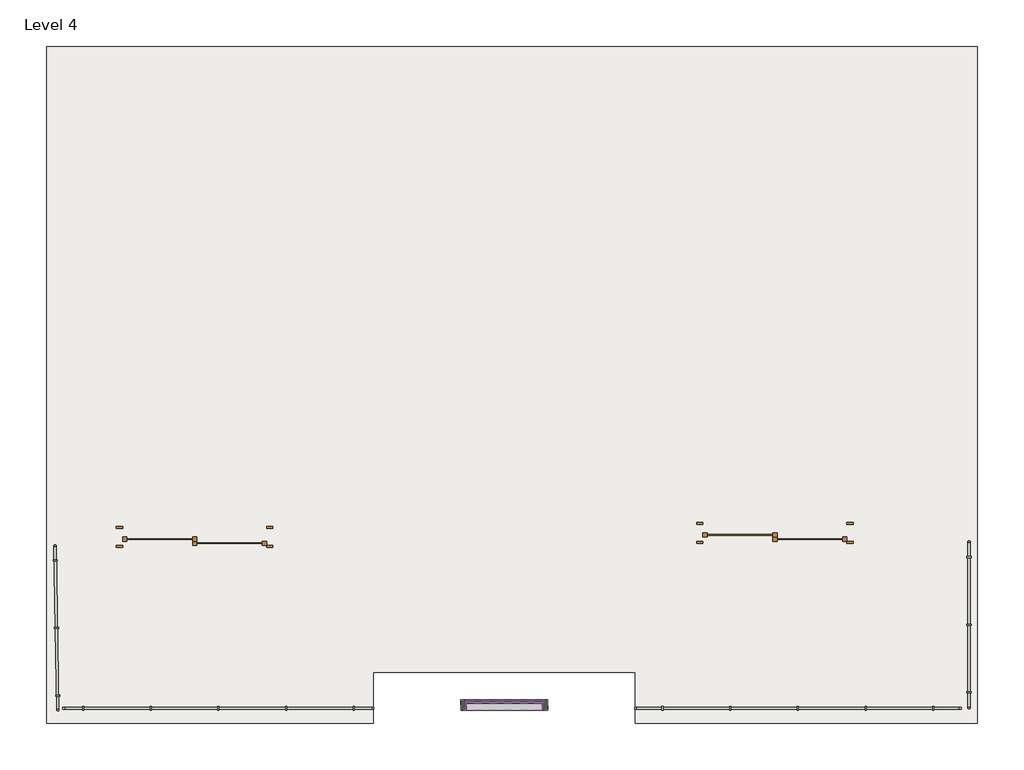
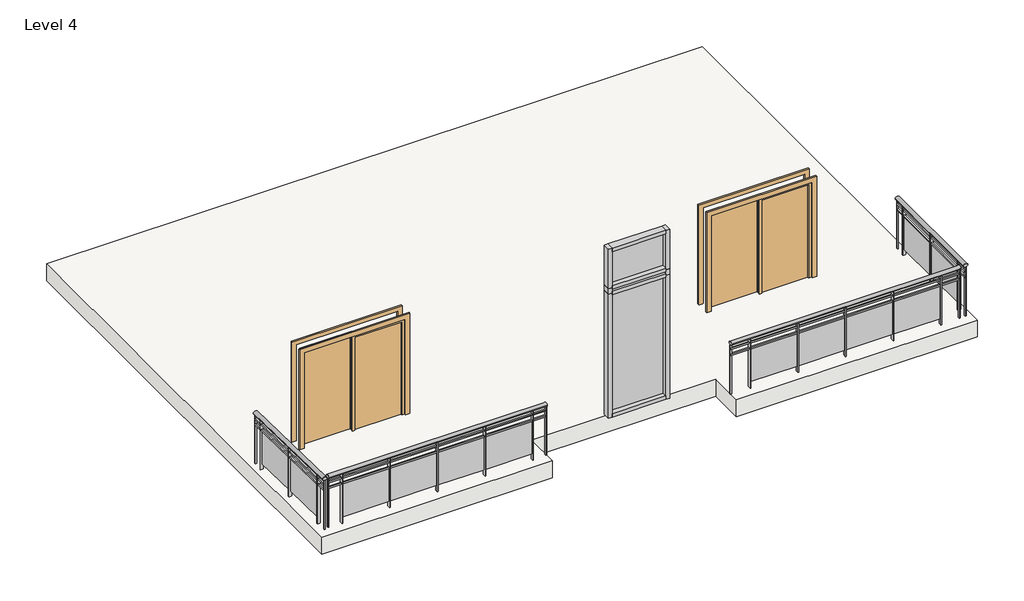
# One storey: 10 members, 4 railings, 3 plates, 2 doors, 1 roof.
"""IFC4 building model written with IfcOpenShell, lengths in millimetres."""

from ifc_helpers import new_model, si_unit, point, frame, origin, place, context, project, spatial, polyline, ellipse_curve, trimmed, outline, extrude, transform, mapped, element, save
from ifc_brep_helpers import plane_surface, extruded_surface, advanced_brep
from components import door_076b30e0, member_d1708325, member_fb13da3b, member_73c23c35, member_410c6227, member_ae70dd35, system_panel_glazed_14bb7e7b, system_panel_glazed_8073c085, system_panel_glazed_7d1a27c5

model = new_model("IFC4")

# Units and contexts
model_context = context("Model", 3, world=origin())
ifc_project = project(units=[si_unit("LENGTHUNIT", "METRE", prefix="MILLI")], contexts=[model_context])

# Site, building, storey
site = spatial("IfcSite", under=ifc_project)
building = spatial("IfcBuilding", under=site)
storey = spatial("IfcBuildingStorey", under=building, Name="Level 4", Elevation=10972.8)

# Doors
placement = place(None, origin())
door_shape = door_076b30e0(model_context)
element("IfcDoor", 1, ObjectType="Door-Double-Sliding : 68\" x 80\"", at=placement, inside=storey, context=model_context, shape_type="MappedRepresentation", body=[
    mapped(door_shape, transform((-2271.8087885, 3717.6236997, 10972.8), x_axis=(-1.0, 0.0, 0.0), y_axis=(0.0, -1.0, 0.0), z_axis=(0.0, 0.0, 1.0))),
])
element("IfcDoor", 2, ObjectType="Door-Double-Sliding : 68\" x 80\"", at=placement, inside=storey, context=model_context, shape_type="MappedRepresentation", body=[
    mapped(door_shape, transform((-9238.1183714, 3666.8236997, 10972.8), x_axis=(-1.0, 0.0, 0.0), y_axis=(0.0, -1.0, 0.0), z_axis=(0.0, 0.0, 1.0))),
])

# Members
member_shape = member_d1708325(model_context)
element("IfcMember", 3, ObjectType="Rectangular Mullion : 2.5\" x 5\" rectangular", at=placement, inside=storey, context=model_context, shape_type="MappedRepresentation", body=[
    mapped(member_shape, transform((-6041.6537147, 1520.5236997, 13817.6), x_axis=(-1.0, 0.0, 0.0), y_axis=(0.0, -1.0, 0.0), z_axis=(0.0, 0.0, 1.0))),
])
member_2_shape = member_fb13da3b(model_context)
element("IfcMember", 4, ObjectType="Rectangular Mullion : 2.5\" x 5\" rectangular", at=placement, inside=storey, context=model_context, shape_type="MappedRepresentation", body=[
    mapped(member_2_shape, transform((-6041.6537147, 1520.5236997, 13919.2), x_axis=(-1.0, 0.0, 0.0), y_axis=(0.0, -1.0, 0.0), z_axis=(0.0, 0.0, 1.0))),
])
member_3_shape = member_73c23c35(model_context)
element("IfcMember", 5, ObjectType="Rectangular Mullion : 2.5\" x 5\" rectangular", at=placement, inside=storey, context=model_context, shape_type="MappedRepresentation", body=[
    mapped(member_3_shape, transform((-5978.1537147, 1520.5236997, 11582.4), x_axis=(0.0, 0.0, -1.0), y_axis=(0.0, -1.0, 0.0), z_axis=(-1.0, 0.0, 0.0))),
])
member_4_shape = member_410c6227(model_context)
element("IfcMember", 6, ObjectType="Rectangular Mullion : 2.5\" x 5\" rectangular", at=placement, inside=storey, context=model_context, shape_type="MappedRepresentation", body=[
    mapped(member_4_shape, transform((-5063.7537147, 1520.5236997, 13817.6), x_axis=(0.0, 0.0, 1.0), y_axis=(0.0, -1.0, 0.0), z_axis=(1.0, 0.0, 0.0))),
])
element("IfcMember", 7, ObjectType="Rectangular Mullion : 2.5\" x 5\" rectangular", at=placement, inside=storey, context=model_context, shape_type="MappedRepresentation", body=[
    mapped(member_4_shape, transform((-5063.7537147, 1520.5236997, 13919.2), x_axis=(0.0, 0.0, 1.0), y_axis=(0.0, -1.0, 0.0), z_axis=(1.0, 0.0, 0.0))),
])
element("IfcMember", 8, ObjectType="Rectangular Mullion : 2.5\" x 5\" rectangular", at=placement, inside=storey, context=model_context, shape_type="MappedRepresentation", body=[
    mapped(member_3_shape, transform((-5063.7537147, 1520.5236997, 14630.4), x_axis=(0.0, 0.0, 1.0), y_axis=(0.0, -1.0, 0.0), z_axis=(1.0, 0.0, 0.0))),
])
element("IfcMember", 9, ObjectType="Rectangular Mullion : 2.5\" x 5\" rectangular", at=placement, inside=storey, context=model_context, shape_type="MappedRepresentation", body=[
    mapped(member_2_shape, transform((-5000.2537147, 1520.5236997, 13817.6), x_axis=(1.0, 0.0, 0.0), y_axis=(0.0, -1.0, 0.0), z_axis=(0.0, 0.0, -1.0))),
])
element("IfcMember", 10, ObjectType="Rectangular Mullion : 2.5\" x 5\" rectangular", at=placement, inside=storey, context=model_context, shape_type="MappedRepresentation", body=[
    mapped(member_shape, transform((-5000.2537147, 1520.5236997, 11582.4), x_axis=(1.0, 0.0, 0.0), y_axis=(0.0, -1.0, 0.0), z_axis=(0.0, 0.0, -1.0))),
])
member_5_shape = member_ae70dd35(model_context)
element("IfcMember", 11, ObjectType="Rectangular Mullion : 2.5\" x 5\" rectangular", at=placement, inside=storey, context=model_context, shape_type="MappedRepresentation", body=[
    mapped(member_5_shape, transform((-6041.6537147, 1520.5236997, 14630.4), x_axis=(-1.0, 0.0, 0.0), y_axis=(0.0, -1.0, 0.0), z_axis=(0.0, 0.0, 1.0))),
])
element("IfcMember", 12, ObjectType="Rectangular Mullion : 2.5\" x 5\" rectangular", at=placement, inside=storey, context=model_context, shape_type="MappedRepresentation", body=[
    mapped(member_5_shape, transform((-5000.2537147, 1520.5236997, 13919.2), x_axis=(1.0, 0.0, 0.0), y_axis=(0.0, -1.0, 0.0), z_axis=(0.0, 0.0, -1.0))),
])

# Plates
system_panel_glazed_shape = system_panel_glazed_14bb7e7b(model_context)
element("IfcPlate", 13, ObjectType="System Panel : Glazed", at=placement, inside=storey, context=model_context, shape_type="MappedRepresentation", body=[
    mapped(system_panel_glazed_shape, transform((-5520.9537147, 1520.5236997, 11645.9), x_axis=(1.0, 0.0, 0.0), y_axis=(0.0, 1.0, 0.0), z_axis=(0.0, 0.0, 1.0))),
])
system_panel_glazed_2_shape = system_panel_glazed_8073c085(model_context)
element("IfcPlate", 14, ObjectType="System Panel : Glazed", at=placement, inside=storey, context=model_context, shape_type="MappedRepresentation", body=[
    mapped(system_panel_glazed_2_shape, transform((-5520.9537147, 1520.5236997, 13849.35), x_axis=(1.0, 0.0, 0.0), y_axis=(0.0, 1.0, 0.0), z_axis=(0.0, 0.0, 1.0))),
])
system_panel_glazed_3_shape = system_panel_glazed_7d1a27c5(model_context)
element("IfcPlate", 15, ObjectType="System Panel : Glazed", at=placement, inside=storey, context=model_context, shape_type="MappedRepresentation", body=[
    mapped(system_panel_glazed_3_shape, transform((-5520.9537147, 1520.5236997, 13950.95), x_axis=(1.0, 0.0, 0.0), y_axis=(0.0, 1.0, 0.0), z_axis=(0.0, 0.0, 1.0))),
])

# Railings
element("IfcRailing", 16, ObjectType="Glass Panel - Bottom Fill", at=placement, inside=storey, context=model_context, shape_type="SolidModel", body=[
    advanced_brep(
    [(-10812.9183714, 1520.5236997, 12192.0), (-10812.9183714, 1444.3236997, 12192.0), (-7091.896639, 1520.5236997, 12192.0), (-7091.896639, 1444.3236997, 12192.0)],
    [
        (0, 1, ellipse_curve(frame((-10812.9183714, 1482.4236997, 12192.0), z_axis=(-1.0, 0.0, 0.0), x_axis=(0.0, -1.0, 0.0)), 38.1, 28.575)),
        (1, 0, ellipse_curve(frame((-10812.9183714, 1482.4236997, 12192.0), z_axis=(-1.0, 0.0, 0.0), x_axis=(0.0, -1.0, 0.0)), 38.1, 28.575)),
        (2, 3, ellipse_curve(frame((-7091.896639, 1482.4236997, 12192.0), z_axis=(1.0, 0.0, 0.0), x_axis=(0.0, -1.0, 0.0)), 38.1, 28.575)),
        (3, 2, ellipse_curve(frame((-7091.896639, 1482.4236997, 12192.0), z_axis=(1.0, 0.0, 0.0), x_axis=(0.0, -1.0, 0.0)), 38.1, 28.575)),
        (0, 2),
        (3, 1),
    ],
    [
        plane_surface(frame((-10812.9183714, 1482.4236997, 12192.0), z_axis=(-1.0, 0.0, 0.0), x_axis=(0.0, 1.0, 0.0))),
        plane_surface(frame((-7091.896639, 1482.4236997, 12192.0), z_axis=(1.0, 0.0, 0.0), x_axis=(0.0, 1.0, 0.0))),
        extruded_surface(trimmed(ellipse_curve(frame((-7091.896639, 1482.4236997, 12192.0), z_axis=(-1.0, 0.0, 0.0), x_axis=(0.0, -1.0, 0.0)), 38.1, 28.575), [point((-7091.896639, 1520.5236997, 12192.0))], [point((-7091.896639, 1444.3236997, 12192.0))], True, "CARTESIAN"), (-3721.0217323999996, 0.0, 0.0), 3721.0217323999996),
        extruded_surface(trimmed(ellipse_curve(frame((-7091.896639, 1482.4236997, 12192.0), z_axis=(-1.0, 0.0, 0.0), x_axis=(0.0, -1.0, 0.0)), 38.1, 28.575), [point((-7091.896639, 1444.3236997, 12192.0))], [point((-7091.896639, 1520.5236997, 12192.0))], True, "CARTESIAN"), (-3721.0217323999996, 0.0, 0.0), 3721.0217323999996),
    ],
    [
        (0, [[1, 2]]),
        (1, [[3, 4]]),
        (2, [[-1, 5, -4, 6]]),
        (3, [[-2, -6, -3, -5]]),
    ],
),
    extrude(outline(polyline([(-10812.9183714, 1469.7236997), (-10812.9183714, 1495.1236997), (-7091.896639, 1495.1236997), (-7091.896639, 1469.7236997), (-10812.9183714, 1469.7236997)])), frame((0.0, 0.0, 12077.7), z_axis=(0.0, 0.0, 1.0), x_axis=(1.0, 0.0, 0.0)), (0.0, 0.0, 1.0), 25.4),
    extrude(outline(polyline([(-10812.9183714, 1469.7236997), (-10812.9183714, 1495.1236997), (-7091.896639, 1495.1236997), (-7091.896639, 1469.7236997), (-10812.9183714, 1469.7236997)])), frame((0.0, 0.0, 11976.1), z_axis=(0.0, 0.0, 1.0), x_axis=(1.0, 0.0, 0.0)), (0.0, 0.0, 1.0), 25.4),
    extrude(outline(polyline([(-7333.1575052, 1457.0236997), (-7333.1575052, 1507.8236997), (-7320.4575052, 1507.8236997), (-7320.4575052, 1457.0236997), (-7333.1575052, 1457.0236997)])), frame((0.0, 0.0, 11277.6), z_axis=(0.0, 0.0, 1.0), x_axis=(1.0, 0.0, 0.0)), (0.0, 0.0, 1.0), 885.6788223),
    extrude(outline(polyline([(-8139.6075052, 1488.9588567), (-7326.8075052, 1488.9588567), (-7326.8075052, 1482.6088567), (-8139.6075052, 1482.6088567), (-8139.6075052, 1488.9588567)])), frame((0.0, 0.0, 11379.2), z_axis=(0.0, 0.0, 1.0), x_axis=(1.0, 0.0, 0.0)), (0.0, 0.0, 1.0), 596.9),
    extrude(outline(polyline([(-8145.9575052, 1457.0236997), (-8145.9575052, 1507.8236997), (-8133.2575052, 1507.8236997), (-8133.2575052, 1457.0236997), (-8145.9575052, 1457.0236997)])), frame((0.0, 0.0, 11277.6), z_axis=(0.0, 0.0, 1.0), x_axis=(1.0, 0.0, 0.0)), (0.0, 0.0, 1.0), 885.6788223),
    extrude(outline(polyline([(-8952.4075052, 1488.9588567), (-8139.6075052, 1488.9588567), (-8139.6075052, 1482.6088567), (-8952.4075052, 1482.6088567), (-8952.4075052, 1488.9588567)])), frame((0.0, 0.0, 11379.2), z_axis=(0.0, 0.0, 1.0), x_axis=(1.0, 0.0, 0.0)), (0.0, 0.0, 1.0), 596.9),
    extrude(outline(polyline([(-8958.7575052, 1457.0236997), (-8958.7575052, 1507.8236997), (-8946.0575052, 1507.8236997), (-8946.0575052, 1457.0236997), (-8958.7575052, 1457.0236997)])), frame((0.0, 0.0, 11277.6), z_axis=(0.0, 0.0, 1.0), x_axis=(1.0, 0.0, 0.0)), (0.0, 0.0, 1.0), 885.6788223),
    extrude(outline(polyline([(-9765.2075052, 1488.9588567), (-8952.4075052, 1488.9588567), (-8952.4075052, 1482.6088567), (-9765.2075052, 1482.6088567), (-9765.2075052, 1488.9588567)])), frame((0.0, 0.0, 11379.2), z_axis=(0.0, 0.0, 1.0), x_axis=(1.0, 0.0, 0.0)), (0.0, 0.0, 1.0), 596.9),
    extrude(outline(polyline([(-9771.5575052, 1457.0236997), (-9771.5575052, 1507.8236997), (-9758.8575052, 1507.8236997), (-9758.8575052, 1457.0236997), (-9771.5575052, 1457.0236997)])), frame((0.0, 0.0, 11277.6), z_axis=(0.0, 0.0, 1.0), x_axis=(1.0, 0.0, 0.0)), (0.0, 0.0, 1.0), 885.6788223),
    extrude(outline(polyline([(-10578.0075052, 1488.9588567), (-9765.2075052, 1488.9588567), (-9765.2075052, 1482.6088567), (-10578.0075052, 1482.6088567), (-10578.0075052, 1488.9588567)])), frame((0.0, 0.0, 11379.2), z_axis=(0.0, 0.0, 1.0), x_axis=(1.0, 0.0, 0.0)), (0.0, 0.0, 1.0), 596.9),
    extrude(outline(polyline([(-10584.3575052, 1457.0236997), (-10584.3575052, 1507.8236997), (-10571.6575052, 1507.8236997), (-10571.6575052, 1457.0236997), (-10584.3575052, 1457.0236997)])), frame((0.0, 0.0, 11277.6), z_axis=(0.0, 0.0, 1.0), x_axis=(1.0, 0.0, 0.0)), (0.0, 0.0, 1.0), 885.6788223),
    extrude(outline(polyline([(-7104.596639, 1472.8986997), (-7104.596639, 1491.9486997), (-7085.546639, 1491.9486997), (-7085.546639, 1472.8986997), (-7104.596639, 1472.8986997)])), frame((0.0, 0.0, 11277.6), z_axis=(0.0, 0.0, 1.0), x_axis=(1.0, 0.0, 0.0)), (0.0, 0.0, 1.0), 885.6788223),
    extrude(outline(polyline([(-10819.2683714, 1472.8986997), (-10819.2683714, 1491.9486997), (-10800.2183714, 1491.9486997), (-10800.2183714, 1472.8986997), (-10819.2683714, 1472.8986997)])), frame((0.0, 0.0, 11277.6), z_axis=(0.0, 0.0, 1.0), x_axis=(1.0, 0.0, 0.0)), (0.0, 0.0, 1.0), 885.6788223),
])
element("IfcRailing", 17, ObjectType="Glass Panel - Bottom Fill", at=placement, inside=storey, context=model_context, shape_type="SolidModel", body=[
    advanced_brep(
    [(-3948.2087885, 1520.5236997, 12192.0), (-3948.2087885, 1444.3236997, 12192.0), (-43.3183714, 1520.5236997, 12192.0), (-43.3183714, 1444.3236997, 12192.0)],
    [
        (0, 1, ellipse_curve(frame((-3948.2087885, 1482.4236997, 12192.0), z_axis=(-1.0, 0.0, 0.0), x_axis=(0.0, -1.0, 0.0)), 38.1, 28.575)),
        (1, 0, ellipse_curve(frame((-3948.2087885, 1482.4236997, 12192.0), z_axis=(-1.0, 0.0, 0.0), x_axis=(0.0, -1.0, 0.0)), 38.1, 28.575)),
        (2, 3, ellipse_curve(frame((-43.3183714, 1482.4236997, 12192.0), z_axis=(1.0, 0.0, 0.0), x_axis=(0.0, -1.0, 0.0)), 38.1, 28.575)),
        (3, 2, ellipse_curve(frame((-43.3183714, 1482.4236997, 12192.0), z_axis=(1.0, 0.0, 0.0), x_axis=(0.0, -1.0, 0.0)), 38.1, 28.575)),
        (0, 2),
        (3, 1),
    ],
    [
        plane_surface(frame((-3948.2087885, 1482.4236997, 12192.0), z_axis=(-1.0, 0.0, 0.0), x_axis=(0.0, 1.0, 0.0))),
        plane_surface(frame((-43.3183714, 1482.4236997, 12192.0), z_axis=(1.0, 0.0, 0.0), x_axis=(0.0, 1.0, 0.0))),
        extruded_surface(trimmed(ellipse_curve(frame((-43.3183714, 1482.4236997, 12192.0), z_axis=(-1.0, 0.0, 0.0), x_axis=(0.0, -1.0, 0.0)), 38.1, 28.575), [point((-43.3183714, 1520.5236997, 12192.0))], [point((-43.3183714, 1444.3236997, 12192.0))], True, "CARTESIAN"), (-3904.8904171, 0.0, 0.0), 3904.8904171),
        extruded_surface(trimmed(ellipse_curve(frame((-43.3183714, 1482.4236997, 12192.0), z_axis=(-1.0, 0.0, 0.0), x_axis=(0.0, -1.0, 0.0)), 38.1, 28.575), [point((-43.3183714, 1444.3236997, 12192.0))], [point((-43.3183714, 1520.5236997, 12192.0))], True, "CARTESIAN"), (-3904.8904171, 0.0, 0.0), 3904.8904171),
    ],
    [
        (0, [[1, 2]]),
        (1, [[3, 4]]),
        (2, [[-1, 5, -4, 6]]),
        (3, [[-2, -6, -3, -5]]),
    ],
),
    extrude(outline(polyline([(-3948.2087885, 1469.7236997), (-3948.2087885, 1495.1236997), (-43.3183714, 1495.1236997), (-43.3183714, 1469.7236997), (-3948.2087885, 1469.7236997)])), frame((0.0, 0.0, 12077.7), z_axis=(0.0, 0.0, 1.0), x_axis=(1.0, 0.0, 0.0)), (0.0, 0.0, 1.0), 25.4),
    extrude(outline(polyline([(-3948.2087885, 1469.7236997), (-3948.2087885, 1495.1236997), (-43.3183714, 1495.1236997), (-43.3183714, 1469.7236997), (-3948.2087885, 1469.7236997)])), frame((0.0, 0.0, 11976.1), z_axis=(0.0, 0.0, 1.0), x_axis=(1.0, 0.0, 0.0)), (0.0, 0.0, 1.0), 25.4),
    extrude(outline(polyline([(-376.51358, 1457.0236997), (-376.51358, 1507.8236997), (-363.81358, 1507.8236997), (-363.81358, 1457.0236997), (-376.51358, 1457.0236997)])), frame((0.0, 0.0, 11277.6), z_axis=(0.0, 0.0, 1.0), x_axis=(1.0, 0.0, 0.0)), (0.0, 0.0, 1.0), 885.6788223),
    extrude(outline(polyline([(-1182.96358, 1488.9588567), (-370.16358, 1488.9588567), (-370.16358, 1482.6088567), (-1182.96358, 1482.6088567), (-1182.96358, 1488.9588567)])), frame((0.0, 0.0, 11379.2), z_axis=(0.0, 0.0, 1.0), x_axis=(1.0, 0.0, 0.0)), (0.0, 0.0, 1.0), 596.9),
    extrude(outline(polyline([(-1189.31358, 1457.0236997), (-1189.31358, 1507.8236997), (-1176.61358, 1507.8236997), (-1176.61358, 1457.0236997), (-1189.31358, 1457.0236997)])), frame((0.0, 0.0, 11277.6), z_axis=(0.0, 0.0, 1.0), x_axis=(1.0, 0.0, 0.0)), (0.0, 0.0, 1.0), 885.6788223),
    extrude(outline(polyline([(-1995.76358, 1488.9588567), (-1182.96358, 1488.9588567), (-1182.96358, 1482.6088567), (-1995.76358, 1482.6088567), (-1995.76358, 1488.9588567)])), frame((0.0, 0.0, 11379.2), z_axis=(0.0, 0.0, 1.0), x_axis=(1.0, 0.0, 0.0)), (0.0, 0.0, 1.0), 596.9),
    extrude(outline(polyline([(-2002.11358, 1457.0236997), (-2002.11358, 1507.8236997), (-1989.41358, 1507.8236997), (-1989.41358, 1457.0236997), (-2002.11358, 1457.0236997)])), frame((0.0, 0.0, 11277.6), z_axis=(0.0, 0.0, 1.0), x_axis=(1.0, 0.0, 0.0)), (0.0, 0.0, 1.0), 885.6788223),
    extrude(outline(polyline([(-2808.56358, 1488.9588567), (-1995.76358, 1488.9588567), (-1995.76358, 1482.6088567), (-2808.56358, 1482.6088567), (-2808.56358, 1488.9588567)])), frame((0.0, 0.0, 11379.2), z_axis=(0.0, 0.0, 1.0), x_axis=(1.0, 0.0, 0.0)), (0.0, 0.0, 1.0), 596.9),
    extrude(outline(polyline([(-2814.91358, 1457.0236997), (-2814.91358, 1507.8236997), (-2802.21358, 1507.8236997), (-2802.21358, 1457.0236997), (-2814.91358, 1457.0236997)])), frame((0.0, 0.0, 11277.6), z_axis=(0.0, 0.0, 1.0), x_axis=(1.0, 0.0, 0.0)), (0.0, 0.0, 1.0), 885.6788223),
    extrude(outline(polyline([(-3621.36358, 1488.9588567), (-2808.56358, 1488.9588567), (-2808.56358, 1482.6088567), (-3621.36358, 1482.6088567), (-3621.36358, 1488.9588567)])), frame((0.0, 0.0, 11379.2), z_axis=(0.0, 0.0, 1.0), x_axis=(1.0, 0.0, 0.0)), (0.0, 0.0, 1.0), 596.9),
    extrude(outline(polyline([(-3627.71358, 1457.0236997), (-3627.71358, 1507.8236997), (-3615.01358, 1507.8236997), (-3615.01358, 1457.0236997), (-3627.71358, 1457.0236997)])), frame((0.0, 0.0, 11277.6), z_axis=(0.0, 0.0, 1.0), x_axis=(1.0, 0.0, 0.0)), (0.0, 0.0, 1.0), 885.6788223),
    extrude(outline(polyline([(-56.0183714, 1472.8986997), (-56.0183714, 1491.9486997), (-36.9683714, 1491.9486997), (-36.9683714, 1472.8986997), (-56.0183714, 1472.8986997)])), frame((0.0, 0.0, 11277.6), z_axis=(0.0, 0.0, 1.0), x_axis=(1.0, 0.0, 0.0)), (0.0, 0.0, 1.0), 885.6788223),
    extrude(outline(polyline([(-3954.5587885, 1472.8986997), (-3954.5587885, 1491.9486997), (-3935.5087885, 1491.9486997), (-3935.5087885, 1472.8986997), (-3954.5587885, 1472.8986997)])), frame((0.0, 0.0, 11277.6), z_axis=(0.0, 0.0, 1.0), x_axis=(1.0, 0.0, 0.0)), (0.0, 0.0, 1.0), 885.6788223),
])
element("IfcRailing", 18, ObjectType="Glass Panel - Bottom Fill", at=placement, inside=storey, context=model_context, shape_type="SolidModel", body=[
    advanced_brep(
    [(-10876.4241743, 3438.8886364, 12192.0), (-10952.6125686, 3437.5587631, 12192.0), (-10841.8474666, 1457.9903828, 12192.0), (-10918.035861, 1456.6605094, 12192.0)],
    [
        (0, 1, ellipse_curve(frame((-10914.5183714, 3438.2236997, 12192.0), z_axis=(-0.01745240643728157, 0.9998476951563913, 0.0), x_axis=(-0.9998476951563913, -0.01745240643728157, 0.0)), 38.1, 28.575)),
        (1, 0, ellipse_curve(frame((-10914.5183714, 3438.2236997, 12192.0), z_axis=(-0.01745240643728157, 0.9998476951563913, 0.0), x_axis=(-0.9998476951563913, -0.01745240643728157, 0.0)), 38.1, 28.575)),
        (2, 3, ellipse_curve(frame((-10879.9416638, 1457.3254461, 12192.0), z_axis=(0.01745240643728157, -0.9998476951563913, 0.0), x_axis=(-0.9998476951563913, -0.01745240643728157, 0.0)), 38.1, 28.575)),
        (3, 2, ellipse_curve(frame((-10879.9416638, 1457.3254461, 12192.0), z_axis=(0.01745240643728157, -0.9998476951563913, 0.0), x_axis=(-0.9998476951563913, -0.01745240643728157, 0.0)), 38.1, 28.575)),
        (0, 2),
        (3, 1),
    ],
    [
        plane_surface(frame((-10914.5183714, 3438.2236997, 12192.0), z_axis=(-0.01745240643728157, 0.9998476951563913, 0.0), x_axis=(0.9998476951563913, 0.01745240643728157, 0.0))),
        plane_surface(frame((-10879.9416638, 1457.3254461, 12192.0), z_axis=(0.01745240643728157, -0.9998476951563913, 0.0), x_axis=(0.9998476951563913, 0.01745240643728157, 0.0))),
        extruded_surface(trimmed(ellipse_curve(frame((-10879.9416638, 1457.3254461, 12192.0), z_axis=(-0.01745240643728157, 0.9998476951563913, 0.0), x_axis=(-0.9998476951563913, -0.01745240643728157, 0.0)), 38.1, 28.575), [point((-10841.8474666, 1457.9903828, 12192.0))], [point((-10918.035861, 1456.6605094, 12192.0))], True, "CARTESIAN"), (-34.57670759999928, 1980.8982536, 0.0), 1981.199999955579),
        extruded_surface(trimmed(ellipse_curve(frame((-10879.9416638, 1457.3254461, 12192.0), z_axis=(-0.01745240643728157, 0.9998476951563913, 0.0), x_axis=(-0.9998476951563913, -0.01745240643728157, 0.0)), 38.1, 28.575), [point((-10918.035861, 1456.6605094, 12192.0))], [point((-10841.8474666, 1457.9903828, 12192.0))], True, "CARTESIAN"), (-34.57670759999928, 1980.8982536, 0.0), 1981.199999955579),
    ],
    [
        (0, [[1, 2]]),
        (1, [[3, 4]]),
        (2, [[-1, 5, -4, 6]]),
        (3, [[-2, -6, -3, -5]]),
    ],
),
    extrude(outline(polyline([(-10927.2164372, 3438.0020542), (-10901.8203057, 3438.4453453), (-10867.2435981, 1457.5470917), (-10892.6397295, 1457.1038005), (-10927.2164372, 3438.0020542)])), frame((0.0, 0.0, 12077.7), z_axis=(0.0, 0.0, 1.0), x_axis=(1.0, 0.0, 0.0)), (0.0, 0.0, 1.0), 25.4),
    extrude(outline(polyline([(-10927.2164372, 3438.0020542), (-10901.8203057, 3438.4453453), (-10867.2435981, 1457.5470917), (-10892.6397295, 1457.1038005), (-10927.2164372, 3438.0020542)])), frame((0.0, 0.0, 11976.1), z_axis=(0.0, 0.0, 1.0), x_axis=(1.0, 0.0, 0.0)), (0.0, 0.0, 1.0), 25.4),
    extrude(outline(polyline([(-10908.5516559, 1641.004108), (-10857.759393, 1641.8906903), (-10857.5377474, 1629.1926246), (-10908.3300103, 1628.3060423), (-10908.5516559, 1641.004108)])), frame((0.0, 0.0, 11277.6), z_axis=(0.0, 0.0, 1.0), x_axis=(1.0, 0.0, 0.0)), (0.0, 0.0, 1.0), 885.6788223),
    extrude(outline(polyline([(-10890.695856, 2447.8886271), (-10876.51054, 1635.2124205), (-10882.8595729, 1635.1015977), (-10897.0448888, 2447.7778044), (-10890.695856, 2447.8886271)])), frame((0.0, 0.0, 11379.2), z_axis=(0.0, 0.0, 1.0), x_axis=(1.0, 0.0, 0.0)), (0.0, 0.0, 1.0), 596.9),
    extrude(outline(polyline([(-10922.7369719, 2453.6803147), (-10871.9447089, 2454.5668969), (-10871.7230634, 2441.8688312), (-10922.5153263, 2440.9822489), (-10922.7369719, 2453.6803147)])), frame((0.0, 0.0, 11277.6), z_axis=(0.0, 0.0, 1.0), x_axis=(1.0, 0.0, 0.0)), (0.0, 0.0, 1.0), 885.6788223),
    extrude(outline(polyline([(-10904.8811719, 3260.5648338), (-10890.695856, 2447.8886271), (-10897.0448888, 2447.7778044), (-10911.2302048, 3260.454011), (-10904.8811719, 3260.5648338)])), frame((0.0, 0.0, 11379.2), z_axis=(0.0, 0.0, 1.0), x_axis=(1.0, 0.0, 0.0)), (0.0, 0.0, 1.0), 596.9),
    extrude(outline(polyline([(-10936.9222878, 3266.3565213), (-10886.1300249, 3267.2431035), (-10885.9083793, 3254.5450378), (-10936.7006423, 3253.6584556), (-10936.9222878, 3266.3565213)])), frame((0.0, 0.0, 11277.6), z_axis=(0.0, 0.0, 1.0), x_axis=(1.0, 0.0, 0.0)), (0.0, 0.0, 1.0), 885.6788223),
    extrude(outline(polyline([(-10889.6868587, 1469.8572777), (-10870.6397601, 1470.189746), (-10870.3072917, 1451.1426474), (-10889.3543903, 1450.8101791), (-10889.6868587, 1469.8572777)])), frame((0.0, 0.0, 11277.6), z_axis=(0.0, 0.0, 1.0), x_axis=(1.0, 0.0, 0.0)), (0.0, 0.0, 1.0), 885.6788223),
    extrude(outline(polyline([(-10924.1527435, 3444.4064984), (-10905.1056449, 3444.7389668), (-10904.7731766, 3425.6918682), (-10923.8202752, 3425.3593998), (-10924.1527435, 3444.4064984)])), frame((0.0, 0.0, 11277.6), z_axis=(0.0, 0.0, 1.0), x_axis=(1.0, 0.0, 0.0)), (0.0, 0.0, 1.0), 885.6788223),
])
element("IfcRailing", 19, ObjectType="Glass Panel - Bottom Fill", at=placement, inside=storey, context=model_context, shape_type="SolidModel", body=[
    advanced_brep(
    [(96.3816286, 3489.0236997, 12192.0), (20.1816286, 3489.0236997, 12192.0), (96.3816286, 1482.4236997, 12192.0), (20.1816286, 1482.4236997, 12192.0)],
    [
        (0, 1, ellipse_curve(frame((58.2816286, 3489.0236997, 12192.0), z_axis=(0.0, 1.0, 0.0), x_axis=(-1.0, 0.0, 0.0)), 38.1, 28.575)),
        (1, 0, ellipse_curve(frame((58.2816286, 3489.0236997, 12192.0), z_axis=(0.0, 1.0, 0.0), x_axis=(-1.0, 0.0, 0.0)), 38.1, 28.575)),
        (2, 3, ellipse_curve(frame((58.2816286, 1482.4236997, 12192.0), z_axis=(0.0, -1.0, 0.0), x_axis=(-1.0, 0.0, 0.0)), 38.1, 28.575)),
        (3, 2, ellipse_curve(frame((58.2816286, 1482.4236997, 12192.0), z_axis=(0.0, -1.0, 0.0), x_axis=(-1.0, 0.0, 0.0)), 38.1, 28.575)),
        (0, 2),
        (3, 1),
    ],
    [
        plane_surface(frame((58.2816286, 3489.0236997, 12192.0), z_axis=(0.0, 1.0, 0.0), x_axis=(0.0, 0.0, -1.0))),
        plane_surface(frame((58.2816286, 1482.4236997, 12192.0), z_axis=(0.0, -1.0, 0.0), x_axis=(0.0, 0.0, -1.0))),
        extruded_surface(trimmed(ellipse_curve(frame((58.2816286, 1482.4236997, 12192.0), z_axis=(0.0, 1.0, 0.0), x_axis=(-1.0, 0.0, 0.0)), 38.1, 28.575), [point((96.3816286, 1482.4236997, 12192.0))], [point((20.1816286, 1482.4236997, 12192.0))], True, "CARTESIAN"), (0.0, 2006.6000000000001, 0.0), 2006.6000000000001),
        extruded_surface(trimmed(ellipse_curve(frame((58.2816286, 1482.4236997, 12192.0), z_axis=(0.0, 1.0, 0.0), x_axis=(-1.0, 0.0, 0.0)), 38.1, 28.575), [point((20.1816286, 1482.4236997, 12192.0))], [point((96.3816286, 1482.4236997, 12192.0))], True, "CARTESIAN"), (0.0, 2006.6000000000001, 0.0), 2006.6000000000001),
    ],
    [
        (0, [[1, 2]]),
        (1, [[3, 4]]),
        (2, [[-1, 5, -4, 6]]),
        (3, [[-2, -6, -3, -5]]),
    ],
),
    extrude(outline(polyline([(45.5816286, 3489.0236997), (70.9816286, 3489.0236997), (70.9816286, 1482.4236997), (45.5816286, 1482.4236997), (45.5816286, 3489.0236997)])), frame((0.0, 0.0, 12077.7), z_axis=(0.0, 0.0, 1.0), x_axis=(1.0, 0.0, 0.0)), (0.0, 0.0, 1.0), 25.4),
    extrude(outline(polyline([(45.5816286, 3489.0236997), (70.9816286, 3489.0236997), (70.9816286, 1482.4236997), (45.5816286, 1482.4236997), (45.5816286, 3489.0236997)])), frame((0.0, 0.0, 11976.1), z_axis=(0.0, 0.0, 1.0), x_axis=(1.0, 0.0, 0.0)), (0.0, 0.0, 1.0), 25.4),
    extrude(outline(polyline([(32.8816286, 1679.2736997), (83.6816286, 1679.2736997), (83.6816286, 1666.5736997), (32.8816286, 1666.5736997), (32.8816286, 1679.2736997)])), frame((0.0, 0.0, 11277.6), z_axis=(0.0, 0.0, 1.0), x_axis=(1.0, 0.0, 0.0)), (0.0, 0.0, 1.0), 885.6788223),
    extrude(outline(polyline([(64.8167856, 2485.7236997), (64.8167856, 1672.9236997), (58.4667856, 1672.9236997), (58.4667856, 2485.7236997), (64.8167856, 2485.7236997)])), frame((0.0, 0.0, 11379.2), z_axis=(0.0, 0.0, 1.0), x_axis=(1.0, 0.0, 0.0)), (0.0, 0.0, 1.0), 596.9),
    extrude(outline(polyline([(32.8816286, 2492.0736997), (83.6816286, 2492.0736997), (83.6816286, 2479.3736997), (32.8816286, 2479.3736997), (32.8816286, 2492.0736997)])), frame((0.0, 0.0, 11277.6), z_axis=(0.0, 0.0, 1.0), x_axis=(1.0, 0.0, 0.0)), (0.0, 0.0, 1.0), 885.6788223),
    extrude(outline(polyline([(64.8167856, 3298.5236997), (64.8167856, 2485.7236997), (58.4667856, 2485.7236997), (58.4667856, 3298.5236997), (64.8167856, 3298.5236997)])), frame((0.0, 0.0, 11379.2), z_axis=(0.0, 0.0, 1.0), x_axis=(1.0, 0.0, 0.0)), (0.0, 0.0, 1.0), 596.9),
    extrude(outline(polyline([(32.8816286, 3304.8736997), (83.6816286, 3304.8736997), (83.6816286, 3292.1736997), (32.8816286, 3292.1736997), (32.8816286, 3304.8736997)])), frame((0.0, 0.0, 11277.6), z_axis=(0.0, 0.0, 1.0), x_axis=(1.0, 0.0, 0.0)), (0.0, 0.0, 1.0), 885.6788223),
    extrude(outline(polyline([(48.7566286, 1495.1236997), (67.8066286, 1495.1236997), (67.8066286, 1476.0736997), (48.7566286, 1476.0736997), (48.7566286, 1495.1236997)])), frame((0.0, 0.0, 11277.6), z_axis=(0.0, 0.0, 1.0), x_axis=(1.0, 0.0, 0.0)), (0.0, 0.0, 1.0), 885.6788223),
    extrude(outline(polyline([(48.7566286, 3495.3736997), (67.8066286, 3495.3736997), (67.8066286, 3476.3236997), (48.7566286, 3476.3236997), (48.7566286, 3495.3736997)])), frame((0.0, 0.0, 11277.6), z_axis=(0.0, 0.0, 1.0), x_axis=(1.0, 0.0, 0.0)), (0.0, 0.0, 1.0), 885.6788223),
])

# Roof
element("IfcRoof", 20, ObjectType="Generic - 12\"", at=placement, inside=storey, context=model_context, shape_type="SweptSolid", body=[
    extrude(outline(polyline([(-11016.1183714, 9432.6236997), (159.8816286, 9432.6236997), (159.8816286, 1304.6236997), (-3948.2087885, 1304.6236997), (-3948.2087885, 1914.2236997), (-7091.896639, 1914.2236997), (-7091.896639, 1304.6236997), (-11016.1183714, 1304.6236997), (-11016.1183714, 9432.6236997)])), frame((0.0, 0.0, 10972.8), z_axis=(0.0, 0.0, 1.0), x_axis=(1.0, 0.0, 0.0)), (0.0, 0.0, 1.0), 304.8),
])

save(model, "model.ifc")

# Revit data of these elements
# Type "Door-Double-Sliding : 68\" x 80\""
#   Type Mark = "11"
#   Construction Type Id = "opn-d45"
#   Assembly Code = "C1020"
#   Analytic Construction = "Wood frame, double glass door "
#   Thickness = 0' - 2"
#   Thermal Resistance (R) = 1.8150 (h·ft²·°F)/BTU
#   Heat Transfer Coefficient (U) = 0.5510 BTU/(h·ft²·°F)
#   Height = 6' - 8"
#   Rail Width = 0' - 2"
#   Stiles = 0' - 2"
#   Trim Projection Ext = 0' - 1"
#   Trim Projection Int = 0' - 1"
#   Trim Width = 0' - 3"
#   Width = 5' - 8"
#   Define Thermal Properties by = 1
#   Glazing = Glass
#   Panel Material = Wood - Birch - Solid Stained Light Low Gloss
#   Trim Material = Paint - Sienna
#   Visual Light Transmittance = 0
#   Solar Heat Gain Coefficient = 0
#   Function = (empty or 0)
#   Wall Closure = (empty or 0)
# Type "Rectangular Mullion : 2.5\" x 5\" rectangular"
#   built-in parameter 1007304 = 0.416667 (stored number, unit not read)
#   built-in parameter 1007301 = 0.104167 (stored number, unit not read)
#   built-in parameter 1007300 = 0.104167 (stored number, unit not read)
# Type "System Panel : Glazed"
#   Construction Type Id = "GSP4R"
#   Analytic Construction = "1/8 in Pilkington single glazing"
#   Visual Light Transmittance = 0.9
#   Solar Heat Gain Coefficient = 0.86
#   Heat Transfer Coefficient (U) = 1.18115 BTU/(h·ft²·°F)
# Type "Glass Panel - Bottom Fill"
#   Assembly Code = "C2010400"
#   built-in parameter 1008612 = 0.0416667 (stored number, unit not read)
#   built-in parameter 1008611 = 0.0416667 (stored number, unit not read)
#   built-in parameter 1008609 = 0.333333 (stored number, unit not read)
#   built-in parameter 1008604 = 0.166667 (stored number, unit not read)
#   built-in parameter 1008603 = 0.166667 (stored number, unit not read)
#   Railing Height = 3' - 0"
#   built-in parameter 1008630 = 2
#   built-in parameter 1008610 = 2
#   built-in parameter 1008618 = Baluster - Square : 3/4"
# Type "Generic - 12\""
#   Assembly Code = "B1020"
#   Layers, outside or top first: 1' - 0" no material (function 1)
# Elements 1, 2 (IfcDoor, "Door-Double-Sliding : 68\" x 80\"")
#   Phase Created = New Construction
#   Materials on its faces: "Paint - Sienna", "Wood - Birch - Solid Stained Light Low Gloss", "Glass"
# Elements 3, 4, 5, 6, 7, 8, 9, 10, 11, 12 (IfcMember, "Rectangular Mullion : 2.5\" x 5\" rectangular")
#   Phase Created = New Construction
#   Materials on its faces: "Aluminum"
# Elements 13, 14, 15 (IfcPlate, "System Panel : Glazed")
#   Phase Created = New Construction
#   Materials on its faces: "Glass"
# Elements 16, 17, 18, 19 (IfcRailing, "Glass Panel - Bottom Fill")
#   built-in parameter 1008621 = 1 (stored number, unit not read)
#   Phase Created = New Construction
#   Materials on its faces: "Glass"
# Element 20 (IfcRoof, "Generic - 12\"")
#   built-in parameter 1001705 = 37 (stored number, unit not read)
#   built-in parameter 1001710 = 33615
#   Phase Created = New Construction
#   Materials on its faces: "Default Roof"
# Materials
#   "Glass": class "Glass", colour RGB 0 128 192, transparency 0.75, Description = "Soda Lime Glass", Cost = 0
#   "Wood - Birch - Solid Stained Light Low Gloss": class "Wood", colour RGB 210 159 95, transparency 0, Cost = 0
#   "Paint - Sienna": colour RGB 118 70 51, transparency 0, Cost = 0
#   "Aluminum": class "Metal", colour RGB 247 247 247, transparency 0, Description = "Aluminum 6061", Cost = 0
#   "Default Roof": colour RGB 88 101 114, transparency 0
